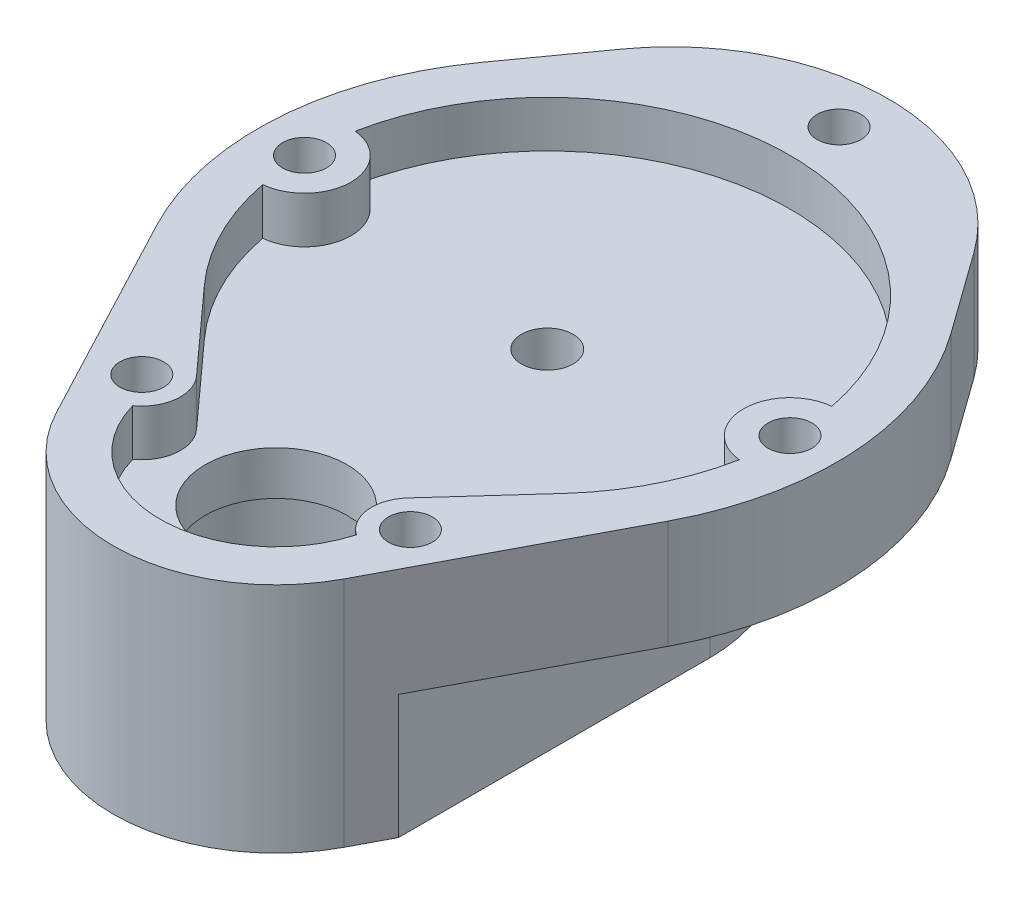
ISO-10303-21;
HEADER;
FILE_DESCRIPTION(('STEP AP214'),'2;1');
FILE_NAME('part.step','',(''),(''),'','','');
FILE_SCHEMA(('AUTOMOTIVE_DESIGN { 1 0 10303 214 1 1 1 1 }'));
ENDSEC;
DATA;
#1=APPLICATION_CONTEXT('core data for automotive mechanical design processes');
#2=APPLICATION_PROTOCOL_DEFINITION('international standard','automotive_design',2000,#1);
#3=PRODUCT_CONTEXT('',#1,'mechanical');
#4=PRODUCT('Part','Part','',(#3));
#5=PRODUCT_RELATED_PRODUCT_CATEGORY('part','',(#4));
#6=PRODUCT_DEFINITION_FORMATION('','',#4);
#7=PRODUCT_DEFINITION_CONTEXT('part definition',#1,'design');
#8=PRODUCT_DEFINITION('design','',#6,#7);
#9=PRODUCT_DEFINITION_SHAPE('','',#8);
#10=(LENGTH_UNIT() NAMED_UNIT(*) SI_UNIT(.MILLI.,.METRE.));
#11=(NAMED_UNIT(*) PLANE_ANGLE_UNIT() SI_UNIT($,.RADIAN.));
#12=(NAMED_UNIT(*) SI_UNIT($,.STERADIAN.) SOLID_ANGLE_UNIT());
#13=UNCERTAINTY_MEASURE_WITH_UNIT(LENGTH_MEASURE(1.E-05),#10,'distance_accuracy_value','');
#14=(GEOMETRIC_REPRESENTATION_CONTEXT(3) GLOBAL_UNCERTAINTY_ASSIGNED_CONTEXT((#13)) GLOBAL_UNIT_ASSIGNED_CONTEXT((#10,
#11,#12)) REPRESENTATION_CONTEXT('',''));
#15=CARTESIAN_POINT('',(0.,0.,0.));
#16=DIRECTION('',(0.,0.,1.));
#17=DIRECTION('',(1.,0.,0.));
#18=AXIS2_PLACEMENT_3D('',#15,#16,#17);
#19=CARTESIAN_POINT('',(0.,0.,0.));
#20=DIRECTION('',(0.,1.,0.));
#21=DIRECTION('',(0.,0.,1.));
#22=AXIS2_PLACEMENT_3D('',#19,#20,#21);
#23=PLANE('',#22);
#24=DIRECTION('',(0.,0.,1.));
#25=VECTOR('',#24,1.);
#26=CARTESIAN_POINT('',(31.5,0.,0.));
#27=LINE('',#26,#25);
#28=CARTESIAN_POINT('',(31.5,0.,-52.5));
#29=VERTEX_POINT('',#28);
#30=CARTESIAN_POINT('',(31.5,0.,7.80075377360281));
#31=VERTEX_POINT('',#30);
#32=EDGE_CURVE('E57',#29,#31,#27,.T.);
#33=ORIENTED_EDGE('',*,*,#32,.F.);
#34=CARTESIAN_POINT('',(0.,0.,-52.5));
#35=DIRECTION('',(0.,-1.,0.));
#36=DIRECTION('',(0.,0.,-1.));
#37=AXIS2_PLACEMENT_3D('',#34,#35,#36);
#38=CIRCLE('',#37,31.5);
#39=CARTESIAN_POINT('',(-31.5,0.,-52.5));
#40=VERTEX_POINT('',#39);
#41=EDGE_CURVE('E393',#40,#29,#38,.T.);
#42=ORIENTED_EDGE('',*,*,#41,.F.);
#43=DIRECTION('',(0.,0.,-1.));
#44=VECTOR('',#43,1.);
#45=CARTESIAN_POINT('',(-31.5,0.,0.));
#46=LINE('',#45,#44);
#47=CARTESIAN_POINT('',(-31.5,0.,7.80075377360279));
#48=VERTEX_POINT('',#47);
#49=EDGE_CURVE('E388',#48,#40,#46,.T.);
#50=ORIENTED_EDGE('',*,*,#49,.F.);
#51=DIRECTION('',(0.466666666666666,0.,0.884433277428107));
#52=VECTOR('',#51,1.);
#53=CARTESIAN_POINT('',(-49.5282635359739,0.,-26.3666666666667));
#54=LINE('',#53,#52);
#55=CARTESIAN_POINT('',(-49.528263535974,0.,-26.3666666666667));
#56=VERTEX_POINT('',#55);
#57=EDGE_CURVE('E344',#56,#48,#54,.T.);
#58=ORIENTED_EDGE('',*,*,#57,.F.);
#59=CARTESIAN_POINT('',(0.,0.,-52.5));
#60=DIRECTION('',(0.,1.,0.));
#61=DIRECTION('',(0.,0.,1.));
#62=AXIS2_PLACEMENT_3D('',#59,#60,#61);
#63=CIRCLE('',#62,56.);
#64=CARTESIAN_POINT('',(-45.4850402757752,0.,-85.1666666666666));
#65=VERTEX_POINT('',#64);
#66=EDGE_CURVE('E370',#65,#56,#63,.T.);
#67=ORIENTED_EDGE('',*,*,#66,.F.);
#68=DIRECTION('',(-0.583333333333332,0.,0.812232862067414));
#69=VECTOR('',#68,1.);
#70=CARTESIAN_POINT('',(-45.4850402757752,0.,-85.1666666666666));
#71=LINE('',#70,#69);
#72=CARTESIAN_POINT('',(-34.1137802068314,0.,-101.));
#73=VERTEX_POINT('',#72);
#74=EDGE_CURVE('E364',#73,#65,#71,.T.);
#75=ORIENTED_EDGE('',*,*,#74,.F.);
#76=CARTESIAN_POINT('',(0.,0.,-76.5));
#77=DIRECTION('',(0.,1.,0.));
#78=DIRECTION('',(0.,0.,1.));
#79=AXIS2_PLACEMENT_3D('',#76,#77,#78);
#80=CIRCLE('',#79,42.);
#81=CARTESIAN_POINT('',(34.1137802068314,0.,-101.));
#82=VERTEX_POINT('',#81);
#83=EDGE_CURVE('E361',#82,#73,#80,.T.);
#84=ORIENTED_EDGE('',*,*,#83,.F.);
#85=DIRECTION('',(-0.583333333333332,0.,-0.812232862067414));
#86=VECTOR('',#85,1.);
#87=CARTESIAN_POINT('',(45.4850402757752,0.,-85.1666666666666));
#88=LINE('',#87,#86);
#89=CARTESIAN_POINT('',(45.4850402757752,0.,-85.1666666666666));
#90=VERTEX_POINT('',#89);
#91=EDGE_CURVE('E363',#90,#82,#88,.T.);
#92=ORIENTED_EDGE('',*,*,#91,.F.);
#93=CARTESIAN_POINT('',(0.,0.,-52.5));
#94=DIRECTION('',(0.,1.,0.));
#95=DIRECTION('',(0.,0.,1.));
#96=AXIS2_PLACEMENT_3D('',#93,#94,#95);
#97=CIRCLE('',#96,56.);
#98=CARTESIAN_POINT('',(49.5282635359739,0.,-26.3666666666667));
#99=VERTEX_POINT('',#98);
#100=EDGE_CURVE('E358',#99,#90,#97,.T.);
#101=ORIENTED_EDGE('',*,*,#100,.F.);
#102=DIRECTION('',(0.466666666666666,0.,-0.884433277428107));
#103=VECTOR('',#102,1.);
#104=CARTESIAN_POINT('',(27.8596482389854,0.,14.7));
#105=LINE('',#104,#103);
#106=EDGE_CURVE('E62',#31,#99,#105,.T.);
#107=ORIENTED_EDGE('',*,*,#106,.F.);
#108=EDGE_LOOP('',(#33,#42,#50,#58,#67,#75,#84,#92,#101,#107));
#109=FACE_BOUND('',#108,.T.);
#110=ADVANCED_FACE('F39',(#109),#23,.F.);
#111=CARTESIAN_POINT('',(0.,21.,0.));
#112=DIRECTION('',(0.,1.,0.));
#113=DIRECTION('',(0.,0.,1.));
#114=AXIS2_PLACEMENT_3D('',#111,#112,#113);
#115=PLANE('',#114);
#116=CARTESIAN_POINT('',(0.,21.,-109.));
#117=DIRECTION('',(0.,1.,0.));
#118=DIRECTION('',(0.,0.,1.));
#119=AXIS2_PLACEMENT_3D('',#116,#117,#118);
#120=CIRCLE('',#119,4.24999999999999);
#121=CARTESIAN_POINT('',(0.,21.,-104.75));
#122=VERTEX_POINT('',#121);
#123=EDGE_CURVE('E224',#122,#122,#120,.T.);
#124=ORIENTED_EDGE('',*,*,#123,.F.);
#125=EDGE_LOOP('',(#124));
#126=FACE_BOUND('',#125,.T.);
#127=CARTESIAN_POINT('',(-47.,21.,-52.5));
#128=DIRECTION('',(0.,1.,0.));
#129=DIRECTION('',(0.,0.,1.));
#130=AXIS2_PLACEMENT_3D('',#127,#128,#129);
#131=CIRCLE('',#130,4.24999999999999);
#132=CARTESIAN_POINT('',(-47.,21.,-48.25));
#133=VERTEX_POINT('',#132);
#134=EDGE_CURVE('E237',#133,#133,#131,.T.);
#135=ORIENTED_EDGE('',*,*,#134,.F.);
#136=EDGE_LOOP('',(#135));
#137=FACE_BOUND('',#136,.T.);
#138=CARTESIAN_POINT('',(47.,21.,-52.5));
#139=DIRECTION('',(0.,1.,0.));
#140=DIRECTION('',(0.,0.,1.));
#141=AXIS2_PLACEMENT_3D('',#138,#139,#140);
#142=CIRCLE('',#141,4.24999999999999);
#143=CARTESIAN_POINT('',(47.,21.,-48.25));
#144=VERTEX_POINT('',#143);
#145=EDGE_CURVE('E244',#144,#144,#142,.T.);
#146=ORIENTED_EDGE('',*,*,#145,.F.);
#147=EDGE_LOOP('',(#146));
#148=FACE_BOUND('',#147,.T.);
#149=CARTESIAN_POINT('',(-26.,21.,0.));
#150=DIRECTION('',(0.,1.,0.));
#151=DIRECTION('',(0.,0.,1.));
#152=AXIS2_PLACEMENT_3D('',#149,#150,#151);
#153=CIRCLE('',#152,4.24999999999999);
#154=CARTESIAN_POINT('',(-26.,21.,4.24999999999999));
#155=VERTEX_POINT('',#154);
#156=EDGE_CURVE('E249',#155,#155,#153,.T.);
#157=ORIENTED_EDGE('',*,*,#156,.F.);
#158=EDGE_LOOP('',(#157));
#159=FACE_BOUND('',#158,.T.);
#160=CARTESIAN_POINT('',(26.,21.,0.));
#161=DIRECTION('',(0.,1.,0.));
#162=DIRECTION('',(0.,0.,1.));
#163=AXIS2_PLACEMENT_3D('',#160,#161,#162);
#164=CIRCLE('',#163,4.24999999999999);
#165=CARTESIAN_POINT('',(26.,21.,4.24999999999999));
#166=VERTEX_POINT('',#165);
#167=EDGE_CURVE('E255',#166,#166,#164,.T.);
#168=ORIENTED_EDGE('',*,*,#167,.F.);
#169=EDGE_LOOP('',(#168));
#170=FACE_BOUND('',#169,.T.);
#171=CARTESIAN_POINT('',(0.,21.,0.));
#172=DIRECTION('',(0.,1.,0.));
#173=DIRECTION('',(0.,0.,1.));
#174=AXIS2_PLACEMENT_3D('',#171,#172,#173);
#175=CIRCLE('',#174,31.5);
#176=CARTESIAN_POINT('',(-27.8596482389854,21.,14.7));
#177=VERTEX_POINT('',#176);
#178=CARTESIAN_POINT('',(27.8596482389854,21.,14.7));
#179=VERTEX_POINT('',#178);
#180=EDGE_CURVE('E336',#177,#179,#175,.T.);
#181=ORIENTED_EDGE('',*,*,#180,.T.);
#182=DIRECTION('',(0.466666666666666,0.,-0.884433277428107));
#183=VECTOR('',#182,1.);
#184=CARTESIAN_POINT('',(27.8596482389854,21.,14.7));
#185=LINE('',#184,#183);
#186=CARTESIAN_POINT('',(49.5282635359739,21.,-26.3666666666667));
#187=VERTEX_POINT('',#186);
#188=EDGE_CURVE('E342',#179,#187,#185,.T.);
#189=ORIENTED_EDGE('',*,*,#188,.T.);
#190=CARTESIAN_POINT('',(0.,21.,-52.5));
#191=DIRECTION('',(0.,1.,0.));
#192=DIRECTION('',(0.,0.,1.));
#193=AXIS2_PLACEMENT_3D('',#190,#191,#192);
#194=CIRCLE('',#193,56.);
#195=CARTESIAN_POINT('',(45.4850402757752,21.,-85.1666666666666));
#196=VERTEX_POINT('',#195);
#197=EDGE_CURVE('E345',#187,#196,#194,.T.);
#198=ORIENTED_EDGE('',*,*,#197,.T.);
#199=DIRECTION('',(-0.583333333333332,0.,-0.812232862067414));
#200=VECTOR('',#199,1.);
#201=CARTESIAN_POINT('',(45.4850402757752,21.,-85.1666666666666));
#202=LINE('',#201,#200);
#203=CARTESIAN_POINT('',(34.1137802068314,21.,-101.));
#204=VERTEX_POINT('',#203);
#205=EDGE_CURVE('E350',#196,#204,#202,.T.);
#206=ORIENTED_EDGE('',*,*,#205,.T.);
#207=CARTESIAN_POINT('',(0.,21.,-76.5));
#208=DIRECTION('',(0.,1.,0.));
#209=DIRECTION('',(0.,0.,1.));
#210=AXIS2_PLACEMENT_3D('',#207,#208,#209);
#211=CIRCLE('',#210,42.);
#212=CARTESIAN_POINT('',(-34.1137802068314,21.,-101.));
#213=VERTEX_POINT('',#212);
#214=EDGE_CURVE('E349',#204,#213,#211,.T.);
#215=ORIENTED_EDGE('',*,*,#214,.T.);
#216=DIRECTION('',(-0.583333333333332,0.,0.812232862067414));
#217=VECTOR('',#216,1.);
#218=CARTESIAN_POINT('',(-45.4850402757752,21.,-85.1666666666666));
#219=LINE('',#218,#217);
#220=CARTESIAN_POINT('',(-45.4850402757752,21.,-85.1666666666666));
#221=VERTEX_POINT('',#220);
#222=EDGE_CURVE('E352',#213,#221,#219,.T.);
#223=ORIENTED_EDGE('',*,*,#222,.T.);
#224=CARTESIAN_POINT('',(0.,21.,-52.5));
#225=DIRECTION('',(0.,1.,0.));
#226=DIRECTION('',(0.,0.,1.));
#227=AXIS2_PLACEMENT_3D('',#224,#225,#226);
#228=CIRCLE('',#227,56.);
#229=CARTESIAN_POINT('',(-49.528263535974,21.,-26.3666666666667));
#230=VERTEX_POINT('',#229);
#231=EDGE_CURVE('E355',#221,#230,#228,.T.);
#232=ORIENTED_EDGE('',*,*,#231,.T.);
#233=DIRECTION('',(0.466666666666666,0.,0.884433277428107));
#234=VECTOR('',#233,1.);
#235=CARTESIAN_POINT('',(-49.5282635359739,21.,-26.3666666666667));
#236=LINE('',#235,#234);
#237=EDGE_CURVE('E353',#230,#177,#236,.T.);
#238=ORIENTED_EDGE('',*,*,#237,.T.);
#239=EDGE_LOOP('',(#181,#189,#198,#206,#215,#223,#232,#238));
#240=FACE_BOUND('',#239,.T.);
#241=CARTESIAN_POINT('',(0.,21.,-52.5));
#242=DIRECTION('',(0.,1.,0.));
#243=DIRECTION('',(0.,0.,1.));
#244=AXIS2_PLACEMENT_3D('',#241,#242,#243);
#245=CIRCLE('',#244,47.);
#246=CARTESIAN_POINT('',(46.1382978723404,21.,-61.458653327548));
#247=VERTEX_POINT('',#246);
#248=CARTESIAN_POINT('',(-46.1382978723404,21.,-61.458653327548));
#249=VERTEX_POINT('',#248);
#250=EDGE_CURVE('E257',#247,#249,#245,.T.);
#251=ORIENTED_EDGE('',*,*,#250,.F.);
#252=CARTESIAN_POINT('',(47.,21.,-52.5));
#253=DIRECTION('',(0.,-1.,0.));
#254=DIRECTION('',(0.,0.,-1.));
#255=AXIS2_PLACEMENT_3D('',#252,#253,#254);
#256=CIRCLE('',#255,8.99999999999997);
#257=CARTESIAN_POINT('',(46.1382978723404,21.,-43.541346672452));
#258=VERTEX_POINT('',#257);
#259=EDGE_CURVE('E264',#258,#247,#256,.T.);
#260=ORIENTED_EDGE('',*,*,#259,.F.);
#261=CARTESIAN_POINT('',(0.,21.,-52.5));
#262=DIRECTION('',(0.,1.,0.));
#263=DIRECTION('',(0.,0.,1.));
#264=AXIS2_PLACEMENT_3D('',#261,#262,#263);
#265=CIRCLE('',#264,47.);
#266=CARTESIAN_POINT('',(34.8564067680253,21.,-20.9717443041649));
#267=VERTEX_POINT('',#266);
#268=EDGE_CURVE('E314',#267,#258,#265,.T.);
#269=ORIENTED_EDGE('',*,*,#268,.F.);
#270=DIRECTION('',(0.670813950975215,0.,-0.741625675915432));
#271=VECTOR('',#270,1.);
#272=CARTESIAN_POINT('',(34.8564067680253,21.,-20.9717443041649));
#273=LINE('',#272,#271);
#274=CARTESIAN_POINT('',(20.4378074306343,21.,-5.03110463231411));
#275=VERTEX_POINT('',#274);
#276=EDGE_CURVE('E313',#275,#267,#273,.T.);
#277=ORIENTED_EDGE('',*,*,#276,.F.);
#278=CARTESIAN_POINT('',(26.,21.,0.));
#279=DIRECTION('',(0.,-1.,0.));
#280=DIRECTION('',(0.,0.,-1.));
#281=AXIS2_PLACEMENT_3D('',#278,#279,#280);
#282=CIRCLE('',#281,7.5);
#283=CARTESIAN_POINT('',(21.6538461538462,21.,6.11236016163659));
#284=VERTEX_POINT('',#283);
#285=EDGE_CURVE('E306',#284,#275,#282,.T.);
#286=ORIENTED_EDGE('',*,*,#285,.F.);
#287=CARTESIAN_POINT('',(0.,21.,0.));
#288=DIRECTION('',(0.,1.,0.));
#289=DIRECTION('',(0.,0.,1.));
#290=AXIS2_PLACEMENT_3D('',#287,#288,#289);
#291=CIRCLE('',#290,22.5);
#292=CARTESIAN_POINT('',(-21.6538461538461,21.,6.11236016163659));
#293=VERTEX_POINT('',#292);
#294=EDGE_CURVE('E305',#293,#284,#291,.T.);
#295=ORIENTED_EDGE('',*,*,#294,.F.);
#296=CARTESIAN_POINT('',(-26.,21.,0.));
#297=DIRECTION('',(0.,-1.,0.));
#298=DIRECTION('',(0.,0.,1.));
#299=AXIS2_PLACEMENT_3D('',#296,#297,#298);
#300=CIRCLE('',#299,7.5);
#301=CARTESIAN_POINT('',(-20.4378074306343,21.,-5.03110463231411));
#302=VERTEX_POINT('',#301);
#303=EDGE_CURVE('E302',#302,#293,#300,.T.);
#304=ORIENTED_EDGE('',*,*,#303,.F.);
#305=DIRECTION('',(0.670813950975215,0.,0.741625675915432));
#306=VECTOR('',#305,1.);
#307=CARTESIAN_POINT('',(-21.5964730043659,21.,-6.3120799877453));
#308=LINE('',#307,#306);
#309=CARTESIAN_POINT('',(-34.8564067680253,21.,-20.9717443041648));
#310=VERTEX_POINT('',#309);
#311=EDGE_CURVE('E296',#310,#302,#308,.T.);
#312=ORIENTED_EDGE('',*,*,#311,.F.);
#313=CARTESIAN_POINT('',(0.,21.,-52.5));
#314=DIRECTION('',(0.,1.,0.));
#315=DIRECTION('',(0.,0.,1.));
#316=AXIS2_PLACEMENT_3D('',#313,#314,#315);
#317=CIRCLE('',#316,47.);
#318=CARTESIAN_POINT('',(-46.1382978723404,21.,-43.541346672452));
#319=VERTEX_POINT('',#318);
#320=EDGE_CURVE('E297',#319,#310,#317,.T.);
#321=ORIENTED_EDGE('',*,*,#320,.F.);
#322=CARTESIAN_POINT('',(-47.,21.,-52.5));
#323=DIRECTION('',(0.,-1.,0.));
#324=DIRECTION('',(0.,0.,1.));
#325=AXIS2_PLACEMENT_3D('',#322,#323,#324);
#326=CIRCLE('',#325,8.99999999999997);
#327=EDGE_CURVE('E291',#249,#319,#326,.T.);
#328=ORIENTED_EDGE('',*,*,#327,.F.);
#329=EDGE_LOOP('',(#251,#260,#269,#277,#286,#295,#304,#312,#321,#328));
#330=FACE_BOUND('',#329,.T.);
#331=ADVANCED_FACE('F460',(#126,#137,#148,#159,#170,#240,#330),#115,.T.);
#332=CARTESIAN_POINT('',(0.,21.,0.));
#333=DIRECTION('',(0.,-1.,0.));
#334=DIRECTION('',(0.,0.,-1.));
#335=AXIS2_PLACEMENT_3D('',#332,#333,#334);
#336=CYLINDRICAL_SURFACE('',#335,31.5);
#337=DIRECTION('',(0.,-1.,0.));
#338=VECTOR('',#337,1.);
#339=CARTESIAN_POINT('',(-27.8596482389854,21.,14.7));
#340=LINE('',#339,#338);
#341=CARTESIAN_POINT('',(-27.8596482389854,-24.,14.7));
#342=VERTEX_POINT('',#341);
#343=EDGE_CURVE('E357',#177,#342,#340,.T.);
#344=ORIENTED_EDGE('',*,*,#343,.T.);
#345=CARTESIAN_POINT('',(0.,-24.,0.));
#346=DIRECTION('',(0.,-1.,0.));
#347=DIRECTION('',(0.,0.,-1.));
#348=AXIS2_PLACEMENT_3D('',#345,#346,#347);
#349=CIRCLE('',#348,31.5);
#350=CARTESIAN_POINT('',(27.8596482389854,-24.,14.7));
#351=VERTEX_POINT('',#350);
#352=EDGE_CURVE('E211',#351,#342,#349,.T.);
#353=ORIENTED_EDGE('',*,*,#352,.F.);
#354=DIRECTION('',(0.,-1.,0.));
#355=VECTOR('',#354,1.);
#356=CARTESIAN_POINT('',(27.8596482389854,21.,14.7));
#357=LINE('',#356,#355);
#358=EDGE_CURVE('E11',#179,#351,#357,.T.);
#359=ORIENTED_EDGE('',*,*,#358,.F.);
#360=ORIENTED_EDGE('',*,*,#180,.F.);
#361=EDGE_LOOP('',(#344,#353,#359,#360));
#362=FACE_BOUND('',#361,.T.);
#363=ADVANCED_FACE('F41',(#362),#336,.T.);
#364=CARTESIAN_POINT('',(27.8596482389854,21.,14.7));
#365=DIRECTION('',(-0.884433277428107,0.,-0.466666666666666));
#366=DIRECTION('',(-0.466666666666666,0.,0.884433277428107));
#367=AXIS2_PLACEMENT_3D('',#364,#365,#366);
#368=PLANE('',#367);
#369=ORIENTED_EDGE('',*,*,#358,.T.);
#370=DIRECTION('',(-0.466666666666666,0.,0.884433277428107));
#371=VECTOR('',#370,1.);
#372=CARTESIAN_POINT('',(27.8596482389854,-24.,14.7));
#373=LINE('',#372,#371);
#374=CARTESIAN_POINT('',(31.5,-24.,7.80075377360281));
#375=VERTEX_POINT('',#374);
#376=EDGE_CURVE('E205',#375,#351,#373,.T.);
#377=ORIENTED_EDGE('',*,*,#376,.F.);
#378=DIRECTION('',(0.,1.,0.));
#379=VECTOR('',#378,1.);
#380=CARTESIAN_POINT('',(31.5,-24.,7.80075377360281));
#381=LINE('',#380,#379);
#382=EDGE_CURVE('E206',#375,#31,#381,.T.);
#383=ORIENTED_EDGE('',*,*,#382,.T.);
#384=ORIENTED_EDGE('',*,*,#106,.T.);
#385=DIRECTION('',(0.,-1.,0.));
#386=VECTOR('',#385,1.);
#387=CARTESIAN_POINT('',(49.5282635359739,21.,-26.3666666666667));
#388=LINE('',#387,#386);
#389=EDGE_CURVE('E48',#187,#99,#388,.T.);
#390=ORIENTED_EDGE('',*,*,#389,.F.);
#391=ORIENTED_EDGE('',*,*,#188,.F.);
#392=EDGE_LOOP('',(#369,#377,#383,#384,#390,#391));
#393=FACE_BOUND('',#392,.T.);
#394=ADVANCED_FACE('F204',(#393),#368,.F.);
#395=CARTESIAN_POINT('',(0.,21.,-52.5));
#396=DIRECTION('',(0.,-1.,0.));
#397=DIRECTION('',(0.,0.,-1.));
#398=AXIS2_PLACEMENT_3D('',#395,#396,#397);
#399=CYLINDRICAL_SURFACE('',#398,56.);
#400=ORIENTED_EDGE('',*,*,#100,.T.);
#401=DIRECTION('',(0.,-1.,0.));
#402=VECTOR('',#401,1.);
#403=CARTESIAN_POINT('',(45.4850402757752,21.,-85.1666666666666));
#404=LINE('',#403,#402);
#405=EDGE_CURVE('E383',#196,#90,#404,.T.);
#406=ORIENTED_EDGE('',*,*,#405,.F.);
#407=ORIENTED_EDGE('',*,*,#197,.F.);
#408=ORIENTED_EDGE('',*,*,#389,.T.);
#409=EDGE_LOOP('',(#400,#406,#407,#408));
#410=FACE_BOUND('',#409,.T.);
#411=ADVANCED_FACE('F452',(#410),#399,.T.);
#412=CARTESIAN_POINT('',(45.4850402757752,21.,-85.1666666666666));
#413=DIRECTION('',(-0.812232862067414,0.,0.583333333333332));
#414=DIRECTION('',(0.583333333333332,0.,0.812232862067415));
#415=AXIS2_PLACEMENT_3D('',#412,#413,#414);
#416=PLANE('',#415);
#417=ORIENTED_EDGE('',*,*,#91,.T.);
#418=DIRECTION('',(0.,-1.,0.));
#419=VECTOR('',#418,1.);
#420=CARTESIAN_POINT('',(34.1137802068314,21.,-101.));
#421=LINE('',#420,#419);
#422=EDGE_CURVE('E381',#204,#82,#421,.T.);
#423=ORIENTED_EDGE('',*,*,#422,.F.);
#424=ORIENTED_EDGE('',*,*,#205,.F.);
#425=ORIENTED_EDGE('',*,*,#405,.T.);
#426=EDGE_LOOP('',(#417,#423,#424,#425));
#427=FACE_BOUND('',#426,.T.);
#428=ADVANCED_FACE('F446',(#427),#416,.F.);
#429=CARTESIAN_POINT('',(0.,21.,-76.5));
#430=DIRECTION('',(0.,-1.,0.));
#431=DIRECTION('',(0.,0.,-1.));
#432=AXIS2_PLACEMENT_3D('',#429,#430,#431);
#433=CYLINDRICAL_SURFACE('',#432,42.);
#434=ORIENTED_EDGE('',*,*,#83,.T.);
#435=DIRECTION('',(0.,-1.,0.));
#436=VECTOR('',#435,1.);
#437=CARTESIAN_POINT('',(-34.1137802068314,21.,-101.));
#438=LINE('',#437,#436);
#439=EDGE_CURVE('E378',#213,#73,#438,.T.);
#440=ORIENTED_EDGE('',*,*,#439,.F.);
#441=ORIENTED_EDGE('',*,*,#214,.F.);
#442=ORIENTED_EDGE('',*,*,#422,.T.);
#443=EDGE_LOOP('',(#434,#440,#441,#442));
#444=FACE_BOUND('',#443,.T.);
#445=ADVANCED_FACE('F443',(#444),#433,.T.);
#446=CARTESIAN_POINT('',(-45.4850402757752,21.,-85.1666666666666));
#447=DIRECTION('',(0.812232862067414,0.,0.583333333333332));
#448=DIRECTION('',(0.583333333333332,0.,-0.812232862067415));
#449=AXIS2_PLACEMENT_3D('',#446,#447,#448);
#450=PLANE('',#449);
#451=ORIENTED_EDGE('',*,*,#74,.T.);
#452=DIRECTION('',(0.,-1.,0.));
#453=VECTOR('',#452,1.);
#454=CARTESIAN_POINT('',(-45.4850402757752,21.,-85.1666666666666));
#455=LINE('',#454,#453);
#456=EDGE_CURVE('E374',#221,#65,#455,.T.);
#457=ORIENTED_EDGE('',*,*,#456,.F.);
#458=ORIENTED_EDGE('',*,*,#222,.F.);
#459=ORIENTED_EDGE('',*,*,#439,.T.);
#460=EDGE_LOOP('',(#451,#457,#458,#459));
#461=FACE_BOUND('',#460,.T.);
#462=ADVANCED_FACE('F439',(#461),#450,.F.);
#463=CARTESIAN_POINT('',(0.,21.,-52.5));
#464=DIRECTION('',(0.,-1.,0.));
#465=DIRECTION('',(0.,0.,-1.));
#466=AXIS2_PLACEMENT_3D('',#463,#464,#465);
#467=CYLINDRICAL_SURFACE('',#466,56.);
#468=ORIENTED_EDGE('',*,*,#66,.T.);
#469=DIRECTION('',(0.,-1.,0.));
#470=VECTOR('',#469,1.);
#471=CARTESIAN_POINT('',(-49.528263535974,21.,-26.3666666666667));
#472=LINE('',#471,#470);
#473=EDGE_CURVE('E375',#230,#56,#472,.T.);
#474=ORIENTED_EDGE('',*,*,#473,.F.);
#475=ORIENTED_EDGE('',*,*,#231,.F.);
#476=ORIENTED_EDGE('',*,*,#456,.T.);
#477=EDGE_LOOP('',(#468,#474,#475,#476));
#478=FACE_BOUND('',#477,.T.);
#479=ADVANCED_FACE('F432',(#478),#467,.T.);
#480=CARTESIAN_POINT('',(-49.5282635359739,21.,-26.3666666666667));
#481=DIRECTION('',(0.884433277428107,0.,-0.466666666666666));
#482=DIRECTION('',(-0.466666666666666,0.,-0.884433277428107));
#483=AXIS2_PLACEMENT_3D('',#480,#481,#482);
#484=PLANE('',#483);
#485=ORIENTED_EDGE('',*,*,#57,.T.);
#486=DIRECTION('',(0.,1.,0.));
#487=VECTOR('',#486,1.);
#488=CARTESIAN_POINT('',(-31.5,-24.,7.80075377360277));
#489=LINE('',#488,#487);
#490=CARTESIAN_POINT('',(-31.5,-24.,7.80075377360277));
#491=VERTEX_POINT('',#490);
#492=EDGE_CURVE('E221',#491,#48,#489,.T.);
#493=ORIENTED_EDGE('',*,*,#492,.F.);
#494=DIRECTION('',(-0.466666666666666,0.,-0.884433277428107));
#495=VECTOR('',#494,1.);
#496=CARTESIAN_POINT('',(-31.5,-24.,7.80075377360277));
#497=LINE('',#496,#495);
#498=EDGE_CURVE('E410',#342,#491,#497,.T.);
#499=ORIENTED_EDGE('',*,*,#498,.F.);
#500=ORIENTED_EDGE('',*,*,#343,.F.);
#501=ORIENTED_EDGE('',*,*,#237,.F.);
#502=ORIENTED_EDGE('',*,*,#473,.T.);
#503=EDGE_LOOP('',(#485,#493,#499,#500,#501,#502));
#504=FACE_BOUND('',#503,.T.);
#505=ADVANCED_FACE('F430',(#504),#484,.F.);
#506=CARTESIAN_POINT('',(0.,12.,-52.5));
#507=DIRECTION('',(0.,1.,0.));
#508=DIRECTION('',(0.,0.,1.));
#509=AXIS2_PLACEMENT_3D('',#506,#507,#508);
#510=CYLINDRICAL_SURFACE('',#509,47.);
#511=ORIENTED_EDGE('',*,*,#250,.T.);
#512=DIRECTION('',(0.,1.,0.));
#513=VECTOR('',#512,1.);
#514=CARTESIAN_POINT('',(-46.1382978723404,12.,-61.458653327548));
#515=LINE('',#514,#513);
#516=CARTESIAN_POINT('',(-46.1382978723404,12.,-61.458653327548));
#517=VERTEX_POINT('',#516);
#518=EDGE_CURVE('E292',#517,#249,#515,.T.);
#519=ORIENTED_EDGE('',*,*,#518,.F.);
#520=CARTESIAN_POINT('',(0.,12.,-52.5));
#521=DIRECTION('',(0.,1.,0.));
#522=DIRECTION('',(0.,0.,1.));
#523=AXIS2_PLACEMENT_3D('',#520,#521,#522);
#524=CIRCLE('',#523,47.);
#525=CARTESIAN_POINT('',(46.1382978723404,12.,-61.458653327548));
#526=VERTEX_POINT('',#525);
#527=EDGE_CURVE('E261',#526,#517,#524,.T.);
#528=ORIENTED_EDGE('',*,*,#527,.F.);
#529=DIRECTION('',(0.,1.,0.));
#530=VECTOR('',#529,1.);
#531=CARTESIAN_POINT('',(46.1382978723404,12.,-61.458653327548));
#532=LINE('',#531,#530);
#533=EDGE_CURVE('E317',#526,#247,#532,.T.);
#534=ORIENTED_EDGE('',*,*,#533,.T.);
#535=EDGE_LOOP('',(#511,#519,#528,#534));
#536=FACE_BOUND('',#535,.T.);
#537=ADVANCED_FACE('F478',(#536),#510,.F.);
#538=CARTESIAN_POINT('',(47.,12.,-52.5));
#539=DIRECTION('',(0.,1.,0.));
#540=DIRECTION('',(0.,0.,1.));
#541=AXIS2_PLACEMENT_3D('',#538,#539,#540);
#542=CYLINDRICAL_SURFACE('',#541,8.99999999999997);
#543=ORIENTED_EDGE('',*,*,#259,.T.);
#544=ORIENTED_EDGE('',*,*,#533,.F.);
#545=CARTESIAN_POINT('',(47.,12.,-52.5));
#546=DIRECTION('',(0.,-1.,0.));
#547=DIRECTION('',(0.,0.,-1.));
#548=AXIS2_PLACEMENT_3D('',#545,#546,#547);
#549=CIRCLE('',#548,8.99999999999997);
#550=CARTESIAN_POINT('',(46.1382978723404,12.,-43.541346672452));
#551=VERTEX_POINT('',#550);
#552=EDGE_CURVE('E289',#551,#526,#549,.T.);
#553=ORIENTED_EDGE('',*,*,#552,.F.);
#554=DIRECTION('',(0.,1.,0.));
#555=VECTOR('',#554,1.);
#556=CARTESIAN_POINT('',(46.1382978723404,12.,-43.541346672452));
#557=LINE('',#556,#555);
#558=EDGE_CURVE('E321',#551,#258,#557,.T.);
#559=ORIENTED_EDGE('',*,*,#558,.T.);
#560=EDGE_LOOP('',(#543,#544,#553,#559));
#561=FACE_BOUND('',#560,.T.);
#562=ADVANCED_FACE('F519',(#561),#542,.T.);
#563=CARTESIAN_POINT('',(0.,12.,-52.5));
#564=DIRECTION('',(0.,1.,0.));
#565=DIRECTION('',(0.,0.,1.));
#566=AXIS2_PLACEMENT_3D('',#563,#564,#565);
#567=CYLINDRICAL_SURFACE('',#566,47.);
#568=ORIENTED_EDGE('',*,*,#268,.T.);
#569=ORIENTED_EDGE('',*,*,#558,.F.);
#570=CARTESIAN_POINT('',(0.,12.,-52.5));
#571=DIRECTION('',(0.,1.,0.));
#572=DIRECTION('',(0.,0.,1.));
#573=AXIS2_PLACEMENT_3D('',#570,#571,#572);
#574=CIRCLE('',#573,47.);
#575=CARTESIAN_POINT('',(34.8564067680253,12.,-20.9717443041649));
#576=VERTEX_POINT('',#575);
#577=EDGE_CURVE('E283',#576,#551,#574,.T.);
#578=ORIENTED_EDGE('',*,*,#577,.F.);
#579=DIRECTION('',(0.,1.,0.));
#580=VECTOR('',#579,1.);
#581=CARTESIAN_POINT('',(34.8564067680253,12.,-20.9717443041649));
#582=LINE('',#581,#580);
#583=EDGE_CURVE('E323',#576,#267,#582,.T.);
#584=ORIENTED_EDGE('',*,*,#583,.T.);
#585=EDGE_LOOP('',(#568,#569,#578,#584));
#586=FACE_BOUND('',#585,.T.);
#587=ADVANCED_FACE('F528',(#586),#567,.F.);
#588=CARTESIAN_POINT('',(34.8564067680253,12.,-20.9717443041649));
#589=DIRECTION('',(0.741625675915432,0.,0.670813950975215));
#590=DIRECTION('',(0.670813950975215,0.,-0.741625675915432));
#591=AXIS2_PLACEMENT_3D('',#588,#589,#590);
#592=PLANE('',#591);
#593=ORIENTED_EDGE('',*,*,#276,.T.);
#594=ORIENTED_EDGE('',*,*,#583,.F.);
#595=DIRECTION('',(0.670813950975215,0.,-0.741625675915432));
#596=VECTOR('',#595,1.);
#597=CARTESIAN_POINT('',(34.8564067680253,12.,-20.9717443041649));
#598=LINE('',#597,#596);
#599=CARTESIAN_POINT('',(20.4378074306343,12.,-5.03110463231411));
#600=VERTEX_POINT('',#599);
#601=EDGE_CURVE('E284',#600,#576,#598,.T.);
#602=ORIENTED_EDGE('',*,*,#601,.F.);
#603=DIRECTION('',(0.,1.,0.));
#604=VECTOR('',#603,1.);
#605=CARTESIAN_POINT('',(20.4378074306343,12.,-5.03110463231411));
#606=LINE('',#605,#604);
#607=EDGE_CURVE('E324',#600,#275,#606,.T.);
#608=ORIENTED_EDGE('',*,*,#607,.T.);
#609=EDGE_LOOP('',(#593,#594,#602,#608));
#610=FACE_BOUND('',#609,.T.);
#611=ADVANCED_FACE('F532',(#610),#592,.F.);
#612=CARTESIAN_POINT('',(26.,12.,0.));
#613=DIRECTION('',(0.,1.,0.));
#614=DIRECTION('',(0.,0.,1.));
#615=AXIS2_PLACEMENT_3D('',#612,#613,#614);
#616=CYLINDRICAL_SURFACE('',#615,7.5);
#617=ORIENTED_EDGE('',*,*,#285,.T.);
#618=ORIENTED_EDGE('',*,*,#607,.F.);
#619=CARTESIAN_POINT('',(26.,12.,0.));
#620=DIRECTION('',(0.,-1.,0.));
#621=DIRECTION('',(0.,0.,-1.));
#622=AXIS2_PLACEMENT_3D('',#619,#620,#621);
#623=CIRCLE('',#622,7.5);
#624=CARTESIAN_POINT('',(21.6538461538462,12.,6.11236016163659));
#625=VERTEX_POINT('',#624);
#626=EDGE_CURVE('E276',#625,#600,#623,.T.);
#627=ORIENTED_EDGE('',*,*,#626,.F.);
#628=DIRECTION('',(0.,1.,0.));
#629=VECTOR('',#628,1.);
#630=CARTESIAN_POINT('',(21.6538461538462,12.,6.11236016163659));
#631=LINE('',#630,#629);
#632=EDGE_CURVE('E330',#625,#284,#631,.T.);
#633=ORIENTED_EDGE('',*,*,#632,.T.);
#634=EDGE_LOOP('',(#617,#618,#627,#633));
#635=FACE_BOUND('',#634,.T.);
#636=ADVANCED_FACE('F542',(#635),#616,.T.);
#637=CARTESIAN_POINT('',(0.,12.,0.));
#638=DIRECTION('',(0.,1.,0.));
#639=DIRECTION('',(0.,0.,1.));
#640=AXIS2_PLACEMENT_3D('',#637,#638,#639);
#641=CYLINDRICAL_SURFACE('',#640,22.5);
#642=ORIENTED_EDGE('',*,*,#294,.T.);
#643=ORIENTED_EDGE('',*,*,#632,.F.);
#644=CARTESIAN_POINT('',(0.,12.,0.));
#645=DIRECTION('',(0.,1.,0.));
#646=DIRECTION('',(0.,0.,1.));
#647=AXIS2_PLACEMENT_3D('',#644,#645,#646);
#648=CIRCLE('',#647,22.5);
#649=CARTESIAN_POINT('',(-21.6538461538461,12.,6.11236016163659));
#650=VERTEX_POINT('',#649);
#651=EDGE_CURVE('E277',#650,#625,#648,.T.);
#652=ORIENTED_EDGE('',*,*,#651,.F.);
#653=DIRECTION('',(0.,1.,0.));
#654=VECTOR('',#653,1.);
#655=CARTESIAN_POINT('',(-21.6538461538461,12.,6.11236016163659));
#656=LINE('',#655,#654);
#657=EDGE_CURVE('E328',#650,#293,#656,.T.);
#658=ORIENTED_EDGE('',*,*,#657,.T.);
#659=EDGE_LOOP('',(#642,#643,#652,#658));
#660=FACE_BOUND('',#659,.T.);
#661=ADVANCED_FACE('F554',(#660),#641,.F.);
#662=CARTESIAN_POINT('',(-26.,12.,0.));
#663=DIRECTION('',(0.,1.,0.));
#664=DIRECTION('',(0.,0.,1.));
#665=AXIS2_PLACEMENT_3D('',#662,#663,#664);
#666=CYLINDRICAL_SURFACE('',#665,7.5);
#667=ORIENTED_EDGE('',*,*,#303,.T.);
#668=ORIENTED_EDGE('',*,*,#657,.F.);
#669=CARTESIAN_POINT('',(-26.,12.,0.));
#670=DIRECTION('',(0.,-1.,0.));
#671=DIRECTION('',(0.,0.,1.));
#672=AXIS2_PLACEMENT_3D('',#669,#670,#671);
#673=CIRCLE('',#672,7.5);
#674=CARTESIAN_POINT('',(-20.4378074306343,12.,-5.03110463231411));
#675=VERTEX_POINT('',#674);
#676=EDGE_CURVE('E272',#675,#650,#673,.T.);
#677=ORIENTED_EDGE('',*,*,#676,.F.);
#678=DIRECTION('',(0.,1.,0.));
#679=VECTOR('',#678,1.);
#680=CARTESIAN_POINT('',(-20.4378074306343,12.,-5.03110463231411));
#681=LINE('',#680,#679);
#682=EDGE_CURVE('E332',#675,#302,#681,.T.);
#683=ORIENTED_EDGE('',*,*,#682,.T.);
#684=EDGE_LOOP('',(#667,#668,#677,#683));
#685=FACE_BOUND('',#684,.T.);
#686=ADVANCED_FACE('F562',(#685),#666,.T.);
#687=CARTESIAN_POINT('',(-21.5964730043659,12.,-6.3120799877453));
#688=DIRECTION('',(-0.741625675915432,0.,0.670813950975215));
#689=DIRECTION('',(0.670813950975215,0.,0.741625675915432));
#690=AXIS2_PLACEMENT_3D('',#687,#688,#689);
#691=PLANE('',#690);
#692=ORIENTED_EDGE('',*,*,#311,.T.);
#693=ORIENTED_EDGE('',*,*,#682,.F.);
#694=DIRECTION('',(0.670813950975215,0.,0.741625675915433));
#695=VECTOR('',#694,1.);
#696=CARTESIAN_POINT('',(-34.8564067680253,12.,-20.9717443041648));
#697=LINE('',#696,#695);
#698=CARTESIAN_POINT('',(-34.8564067680253,12.,-20.9717443041648));
#699=VERTEX_POINT('',#698);
#700=EDGE_CURVE('E271',#699,#675,#697,.T.);
#701=ORIENTED_EDGE('',*,*,#700,.F.);
#702=DIRECTION('',(0.,1.,0.));
#703=VECTOR('',#702,1.);
#704=CARTESIAN_POINT('',(-34.8564067680253,12.,-20.9717443041648));
#705=LINE('',#704,#703);
#706=EDGE_CURVE('E334',#699,#310,#705,.T.);
#707=ORIENTED_EDGE('',*,*,#706,.T.);
#708=EDGE_LOOP('',(#692,#693,#701,#707));
#709=FACE_BOUND('',#708,.T.);
#710=ADVANCED_FACE('F572',(#709),#691,.F.);
#711=CARTESIAN_POINT('',(0.,12.,-52.5));
#712=DIRECTION('',(0.,1.,0.));
#713=DIRECTION('',(0.,0.,1.));
#714=AXIS2_PLACEMENT_3D('',#711,#712,#713);
#715=CYLINDRICAL_SURFACE('',#714,47.);
#716=ORIENTED_EDGE('',*,*,#320,.T.);
#717=ORIENTED_EDGE('',*,*,#706,.F.);
#718=CARTESIAN_POINT('',(0.,12.,-52.5));
#719=DIRECTION('',(0.,1.,0.));
#720=DIRECTION('',(0.,0.,1.));
#721=AXIS2_PLACEMENT_3D('',#718,#719,#720);
#722=CIRCLE('',#721,47.);
#723=CARTESIAN_POINT('',(-46.1382978723404,12.,-43.541346672452));
#724=VERTEX_POINT('',#723);
#725=EDGE_CURVE('E268',#724,#699,#722,.T.);
#726=ORIENTED_EDGE('',*,*,#725,.F.);
#727=DIRECTION('',(0.,1.,0.));
#728=VECTOR('',#727,1.);
#729=CARTESIAN_POINT('',(-46.1382978723404,12.,-43.541346672452));
#730=LINE('',#729,#728);
#731=EDGE_CURVE('E333',#724,#319,#730,.T.);
#732=ORIENTED_EDGE('',*,*,#731,.T.);
#733=EDGE_LOOP('',(#716,#717,#726,#732));
#734=FACE_BOUND('',#733,.T.);
#735=ADVANCED_FACE('F583',(#734),#715,.F.);
#736=CARTESIAN_POINT('',(-47.,12.,-52.5));
#737=DIRECTION('',(0.,1.,0.));
#738=DIRECTION('',(0.,0.,1.));
#739=AXIS2_PLACEMENT_3D('',#736,#737,#738);
#740=CYLINDRICAL_SURFACE('',#739,8.99999999999997);
#741=ORIENTED_EDGE('',*,*,#327,.T.);
#742=ORIENTED_EDGE('',*,*,#731,.F.);
#743=CARTESIAN_POINT('',(-47.,12.,-52.5));
#744=DIRECTION('',(0.,-1.,0.));
#745=DIRECTION('',(0.,0.,1.));
#746=AXIS2_PLACEMENT_3D('',#743,#744,#745);
#747=CIRCLE('',#746,8.99999999999997);
#748=EDGE_CURVE('E262',#517,#724,#747,.T.);
#749=ORIENTED_EDGE('',*,*,#748,.F.);
#750=ORIENTED_EDGE('',*,*,#518,.T.);
#751=EDGE_LOOP('',(#741,#742,#749,#750));
#752=FACE_BOUND('',#751,.T.);
#753=ADVANCED_FACE('F589',(#752),#740,.T.);
#754=CARTESIAN_POINT('',(0.,12.,-52.5));
#755=DIRECTION('',(0.,1.,0.));
#756=DIRECTION('',(0.,0.,1.));
#757=AXIS2_PLACEMENT_3D('',#754,#755,#756);
#758=PLANE('',#757);
#759=CARTESIAN_POINT('',(0.,12.,-52.5));
#760=DIRECTION('',(0.,1.,0.));
#761=DIRECTION('',(0.,0.,1.));
#762=AXIS2_PLACEMENT_3D('',#759,#760,#761);
#763=CIRCLE('',#762,5.00000000000001);
#764=CARTESIAN_POINT('',(0.,12.,-47.5));
#765=VERTEX_POINT('',#764);
#766=EDGE_CURVE('E43',#765,#765,#763,.T.);
#767=ORIENTED_EDGE('',*,*,#766,.F.);
#768=EDGE_LOOP('',(#767));
#769=FACE_BOUND('',#768,.T.);
#770=CARTESIAN_POINT('',(0.,12.,0.));
#771=DIRECTION('',(0.,1.,0.));
#772=DIRECTION('',(0.,0.,1.));
#773=AXIS2_PLACEMENT_3D('',#770,#771,#772);
#774=CIRCLE('',#773,13.75);
#775=CARTESIAN_POINT('',(0.,12.,13.75));
#776=VERTEX_POINT('',#775);
#777=EDGE_CURVE('E389',#776,#776,#774,.T.);
#778=ORIENTED_EDGE('',*,*,#777,.F.);
#779=EDGE_LOOP('',(#778));
#780=FACE_BOUND('',#779,.T.);
#781=ORIENTED_EDGE('',*,*,#527,.T.);
#782=ORIENTED_EDGE('',*,*,#748,.T.);
#783=ORIENTED_EDGE('',*,*,#725,.T.);
#784=ORIENTED_EDGE('',*,*,#700,.T.);
#785=ORIENTED_EDGE('',*,*,#676,.T.);
#786=ORIENTED_EDGE('',*,*,#651,.T.);
#787=ORIENTED_EDGE('',*,*,#626,.T.);
#788=ORIENTED_EDGE('',*,*,#601,.T.);
#789=ORIENTED_EDGE('',*,*,#577,.T.);
#790=ORIENTED_EDGE('',*,*,#552,.T.);
#791=EDGE_LOOP('',(#781,#782,#783,#784,#785,#786,#787,#788,#789,#790));
#792=FACE_BOUND('',#791,.T.);
#793=ADVANCED_FACE('F600',(#769,#780,#792),#758,.T.);
#794=CARTESIAN_POINT('',(26.,7.,0.));
#795=DIRECTION('',(0.,1.,0.));
#796=DIRECTION('',(0.,0.,1.));
#797=AXIS2_PLACEMENT_3D('',#794,#795,#796);
#798=CONICAL_SURFACE('',#797,4.24999999999999,1.02974425867665);
#799=CARTESIAN_POINT('',(26.,4.44634236913287,0.));
#800=VERTEX_POINT('',#799);
#801=VERTEX_LOOP('',#800);
#802=FACE_BOUND('',#801,.T.);
#803=CARTESIAN_POINT('',(26.,7.,0.));
#804=DIRECTION('',(0.,1.,0.));
#805=DIRECTION('',(0.,0.,1.));
#806=AXIS2_PLACEMENT_3D('',#803,#804,#805);
#807=CIRCLE('',#806,4.24999999999999);
#808=CARTESIAN_POINT('',(26.,7.,4.24999999999999));
#809=VERTEX_POINT('',#808);
#810=EDGE_CURVE('E260',#809,#809,#807,.T.);
#811=ORIENTED_EDGE('',*,*,#810,.T.);
#812=EDGE_LOOP('',(#811));
#813=FACE_BOUND('',#812,.T.);
#814=ADVANCED_FACE('F606',(#802,#813),#798,.F.);
#815=CARTESIAN_POINT('',(26.,21.,0.));
#816=DIRECTION('',(0.,1.,0.));
#817=DIRECTION('',(0.,0.,1.));
#818=AXIS2_PLACEMENT_3D('',#815,#816,#817);
#819=CYLINDRICAL_SURFACE('',#818,4.24999999999999);
#820=ORIENTED_EDGE('',*,*,#810,.F.);
#821=EDGE_LOOP('',(#820));
#822=FACE_BOUND('',#821,.T.);
#823=ORIENTED_EDGE('',*,*,#167,.T.);
#824=EDGE_LOOP('',(#823));
#825=FACE_BOUND('',#824,.T.);
#826=ADVANCED_FACE('F615',(#822,#825),#819,.F.);
#827=CARTESIAN_POINT('',(-26.,7.,0.));
#828=DIRECTION('',(0.,1.,0.));
#829=DIRECTION('',(0.,0.,1.));
#830=AXIS2_PLACEMENT_3D('',#827,#828,#829);
#831=CONICAL_SURFACE('',#830,4.24999999999999,1.02974425867665);
#832=CARTESIAN_POINT('',(-26.,4.44634236913287,0.));
#833=VERTEX_POINT('',#832);
#834=VERTEX_LOOP('',#833);
#835=FACE_BOUND('',#834,.T.);
#836=CARTESIAN_POINT('',(-26.,7.,0.));
#837=DIRECTION('',(0.,1.,0.));
#838=DIRECTION('',(0.,0.,1.));
#839=AXIS2_PLACEMENT_3D('',#836,#837,#838);
#840=CIRCLE('',#839,4.24999999999999);
#841=CARTESIAN_POINT('',(-26.,7.,4.24999999999999));
#842=VERTEX_POINT('',#841);
#843=EDGE_CURVE('E253',#842,#842,#840,.T.);
#844=ORIENTED_EDGE('',*,*,#843,.T.);
#845=EDGE_LOOP('',(#844));
#846=FACE_BOUND('',#845,.T.);
#847=ADVANCED_FACE('F625',(#835,#846),#831,.F.);
#848=CARTESIAN_POINT('',(-26.,21.,0.));
#849=DIRECTION('',(0.,1.,0.));
#850=DIRECTION('',(0.,0.,1.));
#851=AXIS2_PLACEMENT_3D('',#848,#849,#850);
#852=CYLINDRICAL_SURFACE('',#851,4.24999999999999);
#853=ORIENTED_EDGE('',*,*,#843,.F.);
#854=EDGE_LOOP('',(#853));
#855=FACE_BOUND('',#854,.T.);
#856=ORIENTED_EDGE('',*,*,#156,.T.);
#857=EDGE_LOOP('',(#856));
#858=FACE_BOUND('',#857,.T.);
#859=ADVANCED_FACE('F631',(#855,#858),#852,.F.);
#860=CARTESIAN_POINT('',(47.,7.,-52.5));
#861=DIRECTION('',(0.,1.,0.));
#862=DIRECTION('',(0.,0.,1.));
#863=AXIS2_PLACEMENT_3D('',#860,#861,#862);
#864=CONICAL_SURFACE('',#863,4.24999999999999,1.02974425867665);
#865=CARTESIAN_POINT('',(47.,4.44634236913287,-52.5));
#866=VERTEX_POINT('',#865);
#867=VERTEX_LOOP('',#866);
#868=FACE_BOUND('',#867,.T.);
#869=CARTESIAN_POINT('',(47.,7.,-52.5));
#870=DIRECTION('',(0.,1.,0.));
#871=DIRECTION('',(0.,0.,1.));
#872=AXIS2_PLACEMENT_3D('',#869,#870,#871);
#873=CIRCLE('',#872,4.24999999999999);
#874=CARTESIAN_POINT('',(47.,7.,-48.25));
#875=VERTEX_POINT('',#874);
#876=EDGE_CURVE('E243',#875,#875,#873,.T.);
#877=ORIENTED_EDGE('',*,*,#876,.T.);
#878=EDGE_LOOP('',(#877));
#879=FACE_BOUND('',#878,.T.);
#880=ADVANCED_FACE('F639',(#868,#879),#864,.F.);
#881=CARTESIAN_POINT('',(47.,21.,-52.5));
#882=DIRECTION('',(0.,1.,0.));
#883=DIRECTION('',(0.,0.,1.));
#884=AXIS2_PLACEMENT_3D('',#881,#882,#883);
#885=CYLINDRICAL_SURFACE('',#884,4.24999999999999);
#886=ORIENTED_EDGE('',*,*,#876,.F.);
#887=EDGE_LOOP('',(#886));
#888=FACE_BOUND('',#887,.T.);
#889=ORIENTED_EDGE('',*,*,#145,.T.);
#890=EDGE_LOOP('',(#889));
#891=FACE_BOUND('',#890,.T.);
#892=ADVANCED_FACE('F647',(#888,#891),#885,.F.);
#893=CARTESIAN_POINT('',(-47.,7.,-52.5));
#894=DIRECTION('',(0.,1.,0.));
#895=DIRECTION('',(0.,0.,1.));
#896=AXIS2_PLACEMENT_3D('',#893,#894,#895);
#897=CONICAL_SURFACE('',#896,4.24999999999999,1.02974425867665);
#898=CARTESIAN_POINT('',(-47.,4.44634236913287,-52.5));
#899=VERTEX_POINT('',#898);
#900=VERTEX_LOOP('',#899);
#901=FACE_BOUND('',#900,.T.);
#902=CARTESIAN_POINT('',(-47.,7.,-52.5));
#903=DIRECTION('',(0.,1.,0.));
#904=DIRECTION('',(0.,0.,1.));
#905=AXIS2_PLACEMENT_3D('',#902,#903,#904);
#906=CIRCLE('',#905,4.24999999999999);
#907=CARTESIAN_POINT('',(-47.,7.,-48.25));
#908=VERTEX_POINT('',#907);
#909=EDGE_CURVE('E239',#908,#908,#906,.T.);
#910=ORIENTED_EDGE('',*,*,#909,.T.);
#911=EDGE_LOOP('',(#910));
#912=FACE_BOUND('',#911,.T.);
#913=ADVANCED_FACE('F657',(#901,#912),#897,.F.);
#914=CARTESIAN_POINT('',(-47.,21.,-52.5));
#915=DIRECTION('',(0.,1.,0.));
#916=DIRECTION('',(0.,0.,1.));
#917=AXIS2_PLACEMENT_3D('',#914,#915,#916);
#918=CYLINDRICAL_SURFACE('',#917,4.24999999999999);
#919=ORIENTED_EDGE('',*,*,#909,.F.);
#920=EDGE_LOOP('',(#919));
#921=FACE_BOUND('',#920,.T.);
#922=ORIENTED_EDGE('',*,*,#134,.T.);
#923=EDGE_LOOP('',(#922));
#924=FACE_BOUND('',#923,.T.);
#925=ADVANCED_FACE('F669',(#921,#924),#918,.F.);
#926=CARTESIAN_POINT('',(0.,7.,-109.));
#927=DIRECTION('',(0.,1.,0.));
#928=DIRECTION('',(0.,0.,1.));
#929=AXIS2_PLACEMENT_3D('',#926,#927,#928);
#930=CONICAL_SURFACE('',#929,4.24999999999999,1.02974425867665);
#931=CARTESIAN_POINT('',(0.,4.44634236913287,-109.));
#932=VERTEX_POINT('',#931);
#933=VERTEX_LOOP('',#932);
#934=FACE_BOUND('',#933,.T.);
#935=CARTESIAN_POINT('',(0.,7.,-109.));
#936=DIRECTION('',(0.,1.,0.));
#937=DIRECTION('',(0.,0.,1.));
#938=AXIS2_PLACEMENT_3D('',#935,#936,#937);
#939=CIRCLE('',#938,4.24999999999999);
#940=CARTESIAN_POINT('',(0.,7.,-104.75));
#941=VERTEX_POINT('',#940);
#942=EDGE_CURVE('E229',#941,#941,#939,.T.);
#943=ORIENTED_EDGE('',*,*,#942,.T.);
#944=EDGE_LOOP('',(#943));
#945=FACE_BOUND('',#944,.T.);
#946=ADVANCED_FACE('F677',(#934,#945),#930,.F.);
#947=CARTESIAN_POINT('',(0.,21.,-109.));
#948=DIRECTION('',(0.,1.,0.));
#949=DIRECTION('',(0.,0.,1.));
#950=AXIS2_PLACEMENT_3D('',#947,#948,#949);
#951=CYLINDRICAL_SURFACE('',#950,4.24999999999999);
#952=ORIENTED_EDGE('',*,*,#942,.F.);
#953=EDGE_LOOP('',(#952));
#954=FACE_BOUND('',#953,.T.);
#955=ORIENTED_EDGE('',*,*,#123,.T.);
#956=EDGE_LOOP('',(#955));
#957=FACE_BOUND('',#956,.T.);
#958=ADVANCED_FACE('F681',(#954,#957),#951,.F.);
#959=CARTESIAN_POINT('',(-31.5,-24.,0.));
#960=DIRECTION('',(1.,0.,0.));
#961=DIRECTION('',(0.,0.,-1.));
#962=AXIS2_PLACEMENT_3D('',#959,#960,#961);
#963=PLANE('',#962);
#964=ORIENTED_EDGE('',*,*,#49,.T.);
#965=DIRECTION('',(0.,1.,0.));
#966=VECTOR('',#965,1.);
#967=CARTESIAN_POINT('',(-31.5,-24.,-52.5));
#968=LINE('',#967,#966);
#969=CARTESIAN_POINT('',(-31.5,-24.,-52.5));
#970=VERTEX_POINT('',#969);
#971=EDGE_CURVE('E228',#970,#40,#968,.T.);
#972=ORIENTED_EDGE('',*,*,#971,.F.);
#973=DIRECTION('',(0.,0.,-1.));
#974=VECTOR('',#973,1.);
#975=CARTESIAN_POINT('',(-31.5,-24.,0.));
#976=LINE('',#975,#974);
#977=EDGE_CURVE('E408',#491,#970,#976,.T.);
#978=ORIENTED_EDGE('',*,*,#977,.F.);
#979=ORIENTED_EDGE('',*,*,#492,.T.);
#980=EDGE_LOOP('',(#964,#972,#978,#979));
#981=FACE_BOUND('',#980,.T.);
#982=ADVANCED_FACE('F425',(#981),#963,.F.);
#983=CARTESIAN_POINT('',(0.,-24.,-52.5));
#984=DIRECTION('',(0.,1.,0.));
#985=DIRECTION('',(0.,0.,1.));
#986=AXIS2_PLACEMENT_3D('',#983,#984,#985);
#987=CYLINDRICAL_SURFACE('',#986,31.5);
#988=ORIENTED_EDGE('',*,*,#41,.T.);
#989=DIRECTION('',(0.,1.,0.));
#990=VECTOR('',#989,1.);
#991=CARTESIAN_POINT('',(31.5,-24.,-52.5));
#992=LINE('',#991,#990);
#993=CARTESIAN_POINT('',(31.5,-24.,-52.5));
#994=VERTEX_POINT('',#993);
#995=EDGE_CURVE('E412',#994,#29,#992,.T.);
#996=ORIENTED_EDGE('',*,*,#995,.F.);
#997=CARTESIAN_POINT('',(0.,-24.,-52.5));
#998=DIRECTION('',(0.,-1.,0.));
#999=DIRECTION('',(0.,0.,-1.));
#1000=AXIS2_PLACEMENT_3D('',#997,#998,#999);
#1001=CIRCLE('',#1000,31.5);
#1002=EDGE_CURVE('E220',#970,#994,#1001,.T.);
#1003=ORIENTED_EDGE('',*,*,#1002,.F.);
#1004=ORIENTED_EDGE('',*,*,#971,.T.);
#1005=EDGE_LOOP('',(#988,#996,#1003,#1004));
#1006=FACE_BOUND('',#1005,.T.);
#1007=ADVANCED_FACE('F420',(#1006),#987,.T.);
#1008=CARTESIAN_POINT('',(31.5,-24.,0.));
#1009=DIRECTION('',(-1.,0.,0.));
#1010=DIRECTION('',(0.,0.,1.));
#1011=AXIS2_PLACEMENT_3D('',#1008,#1009,#1010);
#1012=PLANE('',#1011);
#1013=ORIENTED_EDGE('',*,*,#32,.T.);
#1014=ORIENTED_EDGE('',*,*,#382,.F.);
#1015=DIRECTION('',(0.,0.,1.));
#1016=VECTOR('',#1015,1.);
#1017=CARTESIAN_POINT('',(31.5,-24.,0.));
#1018=LINE('',#1017,#1016);
#1019=EDGE_CURVE('E215',#994,#375,#1018,.T.);
#1020=ORIENTED_EDGE('',*,*,#1019,.F.);
#1021=ORIENTED_EDGE('',*,*,#995,.T.);
#1022=EDGE_LOOP('',(#1013,#1014,#1020,#1021));
#1023=FACE_BOUND('',#1022,.T.);
#1024=ADVANCED_FACE('F225',(#1023),#1012,.F.);
#1025=CARTESIAN_POINT('',(0.,-24.,0.));
#1026=DIRECTION('',(0.,-1.,0.));
#1027=DIRECTION('',(0.,0.,-1.));
#1028=AXIS2_PLACEMENT_3D('',#1025,#1026,#1027);
#1029=PLANE('',#1028);
#1030=CARTESIAN_POINT('',(0.,-24.,-52.5));
#1031=DIRECTION('',(0.,-1.,0.));
#1032=DIRECTION('',(0.,0.,-1.));
#1033=AXIS2_PLACEMENT_3D('',#1030,#1031,#1032);
#1034=CIRCLE('',#1033,13.);
#1035=CARTESIAN_POINT('',(0.,-24.,-65.5));
#1036=VERTEX_POINT('',#1035);
#1037=EDGE_CURVE('E856',#1036,#1036,#1034,.T.);
#1038=ORIENTED_EDGE('',*,*,#1037,.F.);
#1039=EDGE_LOOP('',(#1038));
#1040=FACE_BOUND('',#1039,.T.);
#1041=CARTESIAN_POINT('',(0.,-24.,0.));
#1042=DIRECTION('',(0.,-1.,0.));
#1043=DIRECTION('',(0.,0.,-1.));
#1044=AXIS2_PLACEMENT_3D('',#1041,#1042,#1043);
#1045=CIRCLE('',#1044,22.5);
#1046=CARTESIAN_POINT('',(0.,-24.,-22.5));
#1047=VERTEX_POINT('',#1046);
#1048=EDGE_CURVE('E401',#1047,#1047,#1045,.T.);
#1049=ORIENTED_EDGE('',*,*,#1048,.F.);
#1050=EDGE_LOOP('',(#1049));
#1051=FACE_BOUND('',#1050,.T.);
#1052=ORIENTED_EDGE('',*,*,#1019,.T.);
#1053=ORIENTED_EDGE('',*,*,#376,.T.);
#1054=ORIENTED_EDGE('',*,*,#352,.T.);
#1055=ORIENTED_EDGE('',*,*,#498,.T.);
#1056=ORIENTED_EDGE('',*,*,#977,.T.);
#1057=ORIENTED_EDGE('',*,*,#1002,.T.);
#1058=EDGE_LOOP('',(#1052,#1053,#1054,#1055,#1056,#1057));
#1059=FACE_BOUND('',#1058,.T.);
#1060=ADVANCED_FACE('F214',(#1040,#1051,#1059),#1029,.T.);
#1061=CARTESIAN_POINT('',(0.,-24.,0.));
#1062=DIRECTION('',(0.,-1.,0.));
#1063=DIRECTION('',(0.,0.,-1.));
#1064=AXIS2_PLACEMENT_3D('',#1061,#1062,#1063);
#1065=CYLINDRICAL_SURFACE('',#1064,13.75);
#1066=ORIENTED_EDGE('',*,*,#777,.T.);
#1067=EDGE_LOOP('',(#1066));
#1068=FACE_BOUND('',#1067,.T.);
#1069=CARTESIAN_POINT('',(0.,3.5,0.));
#1070=DIRECTION('',(0.,-1.,0.));
#1071=DIRECTION('',(0.,0.,-1.));
#1072=AXIS2_PLACEMENT_3D('',#1069,#1070,#1071);
#1073=CIRCLE('',#1072,13.75);
#1074=CARTESIAN_POINT('',(0.,3.5,-13.75));
#1075=VERTEX_POINT('',#1074);
#1076=EDGE_CURVE('E392',#1075,#1075,#1073,.T.);
#1077=ORIENTED_EDGE('',*,*,#1076,.T.);
#1078=EDGE_LOOP('',(#1077));
#1079=FACE_BOUND('',#1078,.T.);
#1080=ADVANCED_FACE('F758',(#1068,#1079),#1065,.F.);
#1081=CARTESIAN_POINT('',(13.75,3.5,0.));
#1082=DIRECTION('',(0.,1.,0.));
#1083=DIRECTION('',(0.,0.,1.));
#1084=AXIS2_PLACEMENT_3D('',#1081,#1082,#1083);
#1085=PLANE('',#1084);
#1086=ORIENTED_EDGE('',*,*,#1076,.F.);
#1087=EDGE_LOOP('',(#1086));
#1088=FACE_BOUND('',#1087,.T.);
#1089=CARTESIAN_POINT('',(0.,3.5,0.));
#1090=DIRECTION('',(0.,-1.,0.));
#1091=DIRECTION('',(0.,0.,-1.));
#1092=AXIS2_PLACEMENT_3D('',#1089,#1090,#1091);
#1093=CIRCLE('',#1092,22.5);
#1094=CARTESIAN_POINT('',(0.,3.5,-22.5));
#1095=VERTEX_POINT('',#1094);
#1096=EDGE_CURVE('E399',#1095,#1095,#1093,.T.);
#1097=ORIENTED_EDGE('',*,*,#1096,.T.);
#1098=EDGE_LOOP('',(#1097));
#1099=FACE_BOUND('',#1098,.T.);
#1100=ADVANCED_FACE('F768',(#1088,#1099),#1085,.F.);
#1101=CARTESIAN_POINT('',(0.,-24.,0.));
#1102=DIRECTION('',(0.,-1.,0.));
#1103=DIRECTION('',(0.,0.,-1.));
#1104=AXIS2_PLACEMENT_3D('',#1101,#1102,#1103);
#1105=CYLINDRICAL_SURFACE('',#1104,22.5);
#1106=ORIENTED_EDGE('',*,*,#1096,.F.);
#1107=EDGE_LOOP('',(#1106));
#1108=FACE_BOUND('',#1107,.T.);
#1109=ORIENTED_EDGE('',*,*,#1048,.T.);
#1110=EDGE_LOOP('',(#1109));
#1111=FACE_BOUND('',#1110,.T.);
#1112=ADVANCED_FACE('F780',(#1108,#1111),#1105,.F.);
#1113=CARTESIAN_POINT('',(0.,-24.,-52.5));
#1114=DIRECTION('',(0.,-1.,0.));
#1115=DIRECTION('',(0.,0.,-1.));
#1116=AXIS2_PLACEMENT_3D('',#1113,#1114,#1115);
#1117=CYLINDRICAL_SURFACE('',#1116,5.00000000000001);
#1118=ORIENTED_EDGE('',*,*,#766,.T.);
#1119=EDGE_LOOP('',(#1118));
#1120=FACE_BOUND('',#1119,.T.);
#1121=CARTESIAN_POINT('',(0.,-14.,-52.5));
#1122=DIRECTION('',(0.,-1.,0.));
#1123=DIRECTION('',(0.,0.,-1.));
#1124=AXIS2_PLACEMENT_3D('',#1121,#1122,#1123);
#1125=CIRCLE('',#1124,5.00000000000001);
#1126=CARTESIAN_POINT('',(0.,-14.,-57.5));
#1127=VERTEX_POINT('',#1126);
#1128=EDGE_CURVE('E848',#1127,#1127,#1125,.T.);
#1129=ORIENTED_EDGE('',*,*,#1128,.T.);
#1130=EDGE_LOOP('',(#1129));
#1131=FACE_BOUND('',#1130,.T.);
#1132=ADVANCED_FACE('F786',(#1120,#1131),#1117,.F.);
#1133=CARTESIAN_POINT('',(5.00000000000002,-14.,-52.5));
#1134=DIRECTION('',(0.,1.,0.));
#1135=DIRECTION('',(0.,0.,1.));
#1136=AXIS2_PLACEMENT_3D('',#1133,#1134,#1135);
#1137=PLANE('',#1136);
#1138=ORIENTED_EDGE('',*,*,#1128,.F.);
#1139=EDGE_LOOP('',(#1138));
#1140=FACE_BOUND('',#1139,.T.);
#1141=CARTESIAN_POINT('',(0.,-14.,-52.5));
#1142=DIRECTION('',(0.,-1.,0.));
#1143=DIRECTION('',(0.,0.,-1.));
#1144=AXIS2_PLACEMENT_3D('',#1141,#1142,#1143);
#1145=CIRCLE('',#1144,13.);
#1146=CARTESIAN_POINT('',(0.,-14.,-65.5));
#1147=VERTEX_POINT('',#1146);
#1148=EDGE_CURVE('E854',#1147,#1147,#1145,.T.);
#1149=ORIENTED_EDGE('',*,*,#1148,.T.);
#1150=EDGE_LOOP('',(#1149));
#1151=FACE_BOUND('',#1150,.T.);
#1152=ADVANCED_FACE('F797',(#1140,#1151),#1137,.F.);
#1153=CARTESIAN_POINT('',(0.,-24.,-52.5));
#1154=DIRECTION('',(0.,-1.,0.));
#1155=DIRECTION('',(0.,0.,-1.));
#1156=AXIS2_PLACEMENT_3D('',#1153,#1154,#1155);
#1157=CYLINDRICAL_SURFACE('',#1156,13.);
#1158=ORIENTED_EDGE('',*,*,#1148,.F.);
#1159=EDGE_LOOP('',(#1158));
#1160=FACE_BOUND('',#1159,.T.);
#1161=ORIENTED_EDGE('',*,*,#1037,.T.);
#1162=EDGE_LOOP('',(#1161));
#1163=FACE_BOUND('',#1162,.T.);
#1164=ADVANCED_FACE('F810',(#1160,#1163),#1157,.F.);
#1165=CLOSED_SHELL('',(#110,#331,#363,#394,#411,#428,#445,#462,#479,#505,#537,#562,#587,#611,
#636,#661,#686,#710,#735,#753,#793,#814,#826,#847,#859,#880,#892,#913,#925,#946,#958,#982,#1007,
#1024,#1060,#1080,#1100,#1112,#1132,#1152,#1164));
#1166=MANIFOLD_SOLID_BREP('B2',#1165);
#1167=ADVANCED_BREP_SHAPE_REPRESENTATION('',(#18,#1166),#14);
#1168=SHAPE_DEFINITION_REPRESENTATION(#9,#1167);
ENDSEC;
END-ISO-10303-21;
